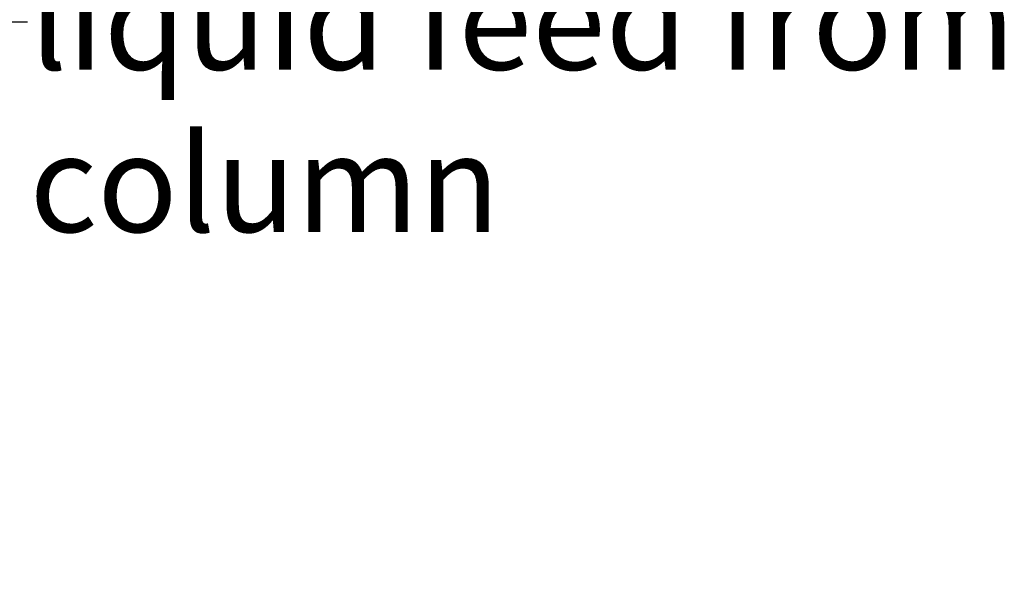
# Model space of a CAD drawing. Units: inches. Extents: x -12 to 334, y -10 to 186.
# Tile 32 of 77: x 152 to 192, y -10 to 14. Entities that reach past the tile are written whole.
import ezdxf
from ezdxf import colors
from ezdxf.entities.mleader import LeaderData, LeaderLine
from ezdxf.math import Vec2, Vec3

# ---------------------------------------------------------------- set-up
doc = ezdxf.new("R2010")
doc.units = ezdxf.units.IN
doc.header["$MEASUREMENT"] = 0
doc.layers.add('M-ANNO-TEXT', color=3, linetype='Continuous', lineweight=25)
doc.styles.get("Standard").update_dxf_attribs({"font": 'arial.ttf'})

msp = doc.modelspace()

# ---------------------------------------------------------------- leaders
at = {"layer": 'M-ANNO-TEXT'}
ml = msp.add_multileader_mtext('Standard', dxfattribs=at)
ml.set_content('liquid feed from\\Pcolumn', color=256)
ml.set_leader_properties()
ml.build(insert=Vec2(0, 0))
ml.multileader.update_dxf_attribs({"dogleg_length": 0.36, "arrow_head_size": 0.7})
ctx = ml.context
ctx.base_point, ctx.arrow_head_size, ctx.landing_gap_size, ctx.plane_origin = Vec3(152.1867, 13.4469), 0.7, 0.09, Vec3(117.7335, 28.8541)
notes = []
notes.append((ctx, [(0, (1, 1, 0), (139.1325, 13.4469), (1, 0), 13.0542, [(0, [(117.7335, 28.8541)], 0, [])])]))
ctx.mtext.insert, ctx.mtext.flow_direction = Vec3(152.2767, 15.4796), 5
for ctx, leaders in notes:
    for number, flags, end, landing, length, lines in leaders:
        leader = LeaderData()
        leader.index, (leader.has_last_leader_line, leader.has_dogleg_vector, leader.attachment_direction) = number, flags
        leader.last_leader_point, leader.dogleg_vector, leader.dogleg_length = Vec3(end), Vec3(landing), length
        for number, points, colour, breaks in lines:
            line = LeaderLine()
            line.index, line.vertices, line.color, line.breaks = number, Vec3.list(points), colors.encode_raw_color(colour), breaks
            leader.lines.append(line)
        ctx.leaders.append(leader)

doc.saveas('drawing.dxf')
